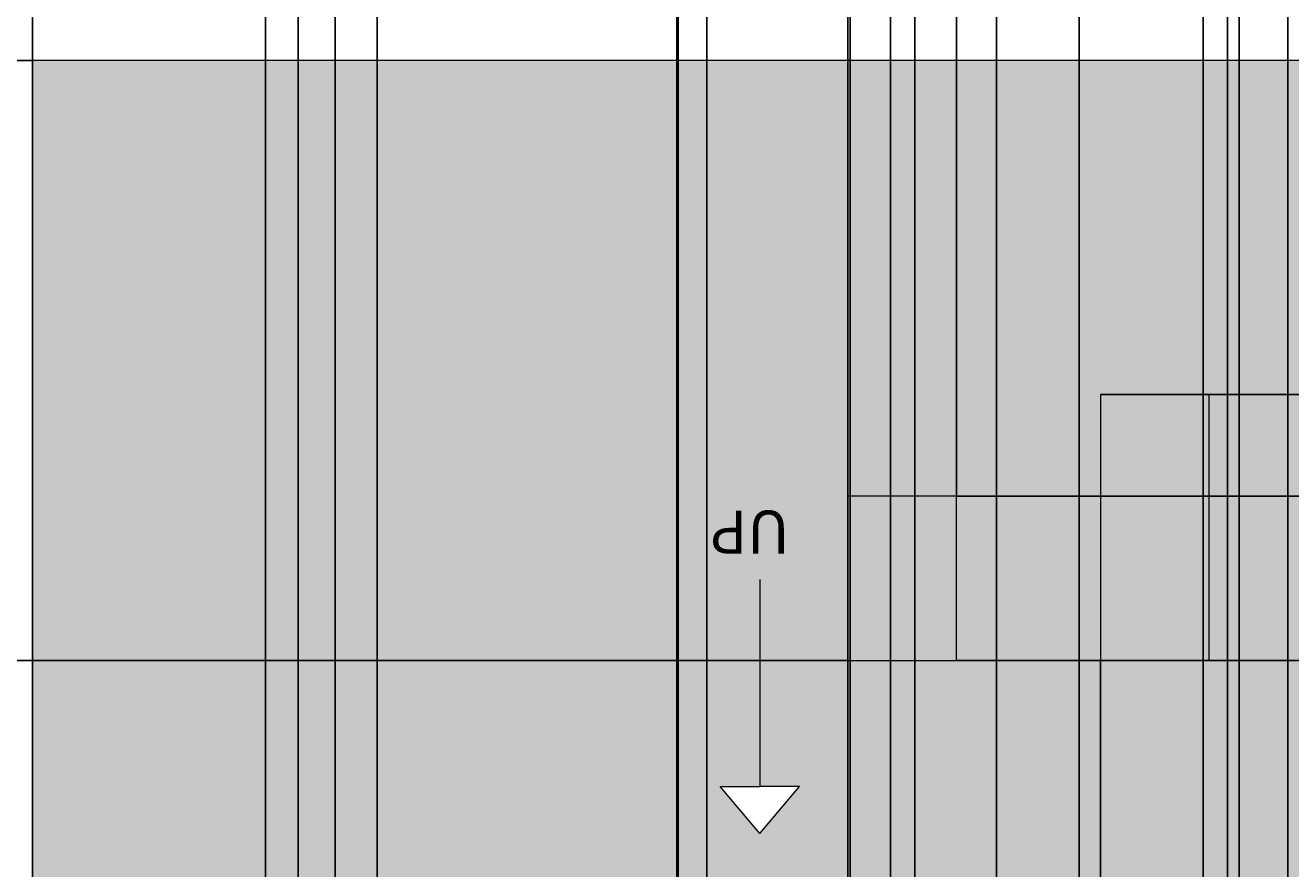
# Model space of a CAD drawing. Units: inches. Extents: x 818 to 1898, y 976 to 2364.
# Tile 78 of 96: x 1083 to 1259, y 2093 to 2211. Entities that reach past the tile are written whole.
import ezdxf

# ---------------------------------------------------------------- set-up
doc = ezdxf.new("R2010")
doc.units = ezdxf.units.IN
doc.header["$LTSCALE"] = 5
doc.header["$MEASUREMENT"] = 0
for name, color, linetype, lineweight in [('A-ANNO-DIMS', 2, 'Continuous', 18), ('A-ANNO-SYMB', 7, 'Continuous', 18), ('A-ANNO-TEXT', 7, 'Continuous', 18), ('L-PAVE', 8, 'Continuous', 18), ('L-PLNT-BEDS', 94, 'Continuous', 18)]:
    doc.layers.add(name, color=color, linetype=linetype, lineweight=lineweight)
doc.layers.add('L-PAVE-PATT', color=9, linetype='Continuous', lineweight=9, true_color=0xc7c8ca)
doc.layers.add('L-PLNT-PATT', color=114, linetype='Continuous', lineweight=9, true_color=0x139b48)
doc.styles.get("Standard").update_dxf_attribs({"font": 'arial.ttf'})
doc.dimstyles.get("Standard").update_dxf_attribs({"dimtxt": 0.18, "dimasz": 0.18, "dimexe": 0.18, "dimexo": 0.0625, "dimgap": 0.09, "dimtad": 0, "dimtih": 1, "dimtoh": 1, "dimdec": 4, "dimzin": 0, "dimdsep": 46, "dimtxsty": 'Standard', "dimcen": 0.09, "dimadec": 0, "dimazin": 0, "dimtfac": 1, "dimtdec": 4, "dimtofl": 0, "dimtmove": 0, "dimatfit": 3, "dimfxl": 1, "dimtolj": 1, "dimtzin": 0, "dimarcsym": 0})

# ---------------------------------------------------------------- blocks, each defined once
blk = doc.blocks.new('*D59')
at = {"layer": 'A-ANNO-DIMS', "color": 0, "lineweight": -2, "ltscale": 5, "transparency": 16777216}
for p, q in [((1251.64, 2300.39), (818.03, 2300.39)), ((818.21, 2300.21), (818.21, 1669.95)), ((818.21, 1039.32), (818.21, 1669.59)), ((896.05, 1039.14), (818.03, 1039.14))]:
    blk.add_line(p, q, dxfattribs=at)
at = {"layer": 'A-ANNO-DIMS', "color": 0, "ltscale": 5, "transparency": 16777216}
for points in [[(818.18, 2300.21), (818.24, 2300.21), (818.21, 2300.39)], [(818.18, 1039.32), (818.24, 1039.32), (818.21, 1039.14)]]:
    blk.add_solid(points, dxfattribs=at)
at = {"layer": 'Defpoints', "color": 0, "ltscale": 5, "transparency": 16777216}
for p in [(818.21, 2300.39), (1251.71, 2300.39), (896.11, 1039.14)]:
    blk.add_point(p, dxfattribs=at)
at = {"layer": 'A-ANNO-DIMS', "color": 0, "ltscale": 5, "transparency": 16777216, "insert": (818.21, 1669.77), "char_height": 0.18, "attachment_point": 5}
blk.add_mtext('\\A1;1261.2', dxfattribs=at)
blk = doc.blocks.new('*D61')
at = {"layer": 'A-ANNO-DIMS', "color": 0, "lineweight": -2, "ltscale": 5, "transparency": 16777216}
for p, q in [((1071.73, 1203.03), (1071.73, 2363.87)), ((1071.91, 2363.69), (1250.94, 2363.69)), ((1430.55, 2363.69), (1251.51, 2363.69)), ((1430.73, 1203.03), (1430.73, 2363.87))]:
    blk.add_line(p, q, dxfattribs=at)
at = {"layer": 'A-ANNO-DIMS', "color": 0, "ltscale": 5, "transparency": 16777216}
for points in [[(1071.91, 2363.72), (1071.91, 2363.66), (1071.73, 2363.69)], [(1430.55, 2363.72), (1430.55, 2363.66), (1430.73, 2363.69)]]:
    blk.add_solid(points, dxfattribs=at)
at = {"layer": 'Defpoints', "color": 0, "ltscale": 5, "transparency": 16777216}
for p in [(1430.73, 2363.69), (1071.73, 1202.96), (1430.73, 1202.96)]:
    blk.add_point(p, dxfattribs=at)
at = {"layer": 'A-ANNO-DIMS', "color": 0, "ltscale": 5, "transparency": 16777216, "insert": (1251.23, 2363.69), "char_height": 0.18, "attachment_point": 5}
blk.add_mtext('\\A1;359', dxfattribs=at)
blk = doc.blocks.new('*D64')
at = {"layer": 'A-ANNO-DIMS', "color": 0, "lineweight": -2, "ltscale": 5, "transparency": 16777216}
for p, q in [((1197.73, 1501.14), (1197.73, 2363.87)), ((1197.91, 2363.69), (1313.93, 2363.69)), ((1430.55, 2363.69), (1314.52, 2363.69)), ((1430.73, 1501.14), (1430.73, 2363.87))]:
    blk.add_line(p, q, dxfattribs=at)
at = {"layer": 'A-ANNO-DIMS', "color": 0, "ltscale": 5, "transparency": 16777216}
for points in [[(1197.91, 2363.72), (1197.91, 2363.66), (1197.73, 2363.69)], [(1430.55, 2363.72), (1430.55, 2363.66), (1430.73, 2363.69)]]:
    blk.add_solid(points, dxfattribs=at)
at = {"layer": 'Defpoints', "color": 0, "ltscale": 5, "transparency": 16777216}
for p in [(1430.73, 2363.69), (1197.73, 1501.08), (1430.73, 1501.08)]:
    blk.add_point(p, dxfattribs=at)
at = {"layer": 'A-ANNO-DIMS', "color": 0, "ltscale": 5, "transparency": 16777216, "insert": (1314.23, 2363.69), "char_height": 0.18, "attachment_point": 5}
blk.add_mtext('\\A1;233', dxfattribs=at)
blk = doc.blocks.new('*D67')
at = {"layer": 'A-ANNO-DIMS', "color": 0, "lineweight": -2, "ltscale": 5, "transparency": 16777216}
for p, q in [((1083.66, 2205.97), (818.03, 2205.97)), ((818.21, 2205.79), (818.21, 2129.71)), ((818.21, 2053.26), (818.21, 2129.34)), ((1083.66, 2053.08), (818.03, 2053.08))]:
    blk.add_line(p, q, dxfattribs=at)
at = {"layer": 'A-ANNO-DIMS', "color": 0, "ltscale": 5, "transparency": 16777216}
for points in [[(818.18, 2205.79), (818.24, 2205.79), (818.21, 2205.97)], [(818.18, 2053.26), (818.24, 2053.26), (818.21, 2053.08)]]:
    blk.add_solid(points, dxfattribs=at)
at = {"layer": 'Defpoints', "color": 0, "ltscale": 5, "transparency": 16777216}
for p in [(818.21, 2205.97), (1083.73, 2205.97), (1083.73, 2053.08)]:
    blk.add_point(p, dxfattribs=at)
at = {"layer": 'A-ANNO-DIMS', "color": 0, "ltscale": 5, "transparency": 16777216, "insert": (818.21, 2129.52), "char_height": 0.18, "attachment_point": 5}
blk.add_mtext('\\A1;152.9', dxfattribs=at)
blk = doc.blocks.new('*D82')
at = {"layer": 'A-ANNO-DIMS', "color": 0, "lineweight": -2, "ltscale": 5, "transparency": 16777216}
for p, q in [((1083.73, 1501.14), (1083.73, 2363.87)), ((1083.91, 2363.69), (1140.45, 2363.69)), ((1197.55, 2363.69), (1141.01, 2363.69)), ((1197.73, 1501.14), (1197.73, 2363.87))]:
    blk.add_line(p, q, dxfattribs=at)
at = {"layer": 'A-ANNO-DIMS', "color": 0, "ltscale": 5, "transparency": 16777216}
for points in [[(1083.91, 2363.72), (1083.91, 2363.66), (1083.73, 2363.69)], [(1197.55, 2363.72), (1197.55, 2363.66), (1197.73, 2363.69)]]:
    blk.add_solid(points, dxfattribs=at)
at = {"layer": 'Defpoints', "color": 0, "ltscale": 5, "transparency": 16777216}
for p in [(1197.73, 2363.69), (1083.73, 1501.08), (1197.73, 1501.08)]:
    blk.add_point(p, dxfattribs=at)
at = {"layer": 'A-ANNO-DIMS', "color": 0, "ltscale": 5, "transparency": 16777216, "insert": (1140.73, 2363.69), "char_height": 0.18, "attachment_point": 5}
blk.add_mtext('\\A1;114', dxfattribs=at)
blk = doc.blocks.new('*D83')
at = {"layer": 'A-ANNO-DIMS', "color": 0, "lineweight": -2, "ltscale": 5, "transparency": 16777216}
for p, q in [((1197.73, 1700.14), (1197.73, 2363.87)), ((1197.91, 2363.69), (1228.02, 2363.69)), ((1258.55, 2363.69), (1228.43, 2363.69)), ((1258.73, 1700.14), (1258.73, 2363.87))]:
    blk.add_line(p, q, dxfattribs=at)
at = {"layer": 'A-ANNO-DIMS', "color": 0, "ltscale": 5, "transparency": 16777216}
for points in [[(1197.91, 2363.72), (1197.91, 2363.66), (1197.73, 2363.69)], [(1258.55, 2363.72), (1258.55, 2363.66), (1258.73, 2363.69)]]:
    blk.add_solid(points, dxfattribs=at)
at = {"layer": 'Defpoints', "color": 0, "ltscale": 5, "transparency": 16777216}
for p in [(1258.73, 2363.69), (1197.73, 1700.08), (1258.73, 1700.08)]:
    blk.add_point(p, dxfattribs=at)
at = {"layer": 'A-ANNO-DIMS', "color": 0, "ltscale": 5, "transparency": 16777216, "insert": (1228.23, 2363.69), "char_height": 0.18, "attachment_point": 5}
blk.add_mtext('\\A1;61', dxfattribs=at)
blk = doc.blocks.new('*D86')
at = {"layer": 'A-ANNO-DIMS', "color": 0, "lineweight": -2, "ltscale": 5, "transparency": 16777216}
for p, q in [((1258.73, 2053.14), (1258.73, 2363.87)), ((1258.91, 2363.69), (1486.43, 2363.69)), ((1714.55, 2363.69), (1487.02, 2363.69)), ((1714.73, 2053.14), (1714.73, 2363.87))]:
    blk.add_line(p, q, dxfattribs=at)
at = {"layer": 'A-ANNO-DIMS', "color": 0, "ltscale": 5, "transparency": 16777216}
for points in [[(1258.91, 2363.72), (1258.91, 2363.66), (1258.73, 2363.69)], [(1714.55, 2363.72), (1714.55, 2363.66), (1714.73, 2363.69)]]:
    blk.add_solid(points, dxfattribs=at)
at = {"layer": 'Defpoints', "color": 0, "ltscale": 5, "transparency": 16777216}
for p in [(1714.73, 2363.69), (1258.73, 2053.08), (1714.73, 2053.08)]:
    blk.add_point(p, dxfattribs=at)
at = {"layer": 'A-ANNO-DIMS', "color": 0, "ltscale": 5, "transparency": 16777216, "insert": (1486.73, 2363.69), "char_height": 0.18, "attachment_point": 5}
blk.add_mtext('\\A1;456', dxfattribs=at)
blk = doc.blocks.new('*D87')
at = {"layer": 'A-ANNO-DIMS', "color": 0, "lineweight": -2, "ltscale": 5, "transparency": 16777216}
for p, q in [((992.73, 2294.28), (992.73, 2363.87)), ((992.91, 2363.69), (1038.02, 2363.69)), ((1083.55, 2363.69), (1038.43, 2363.69)), ((1083.73, 2206.03), (1083.73, 2363.87))]:
    blk.add_line(p, q, dxfattribs=at)
at = {"layer": 'A-ANNO-DIMS', "color": 0, "ltscale": 5, "transparency": 16777216}
for points in [[(992.91, 2363.72), (992.91, 2363.66), (992.73, 2363.69)], [(1083.55, 2363.72), (1083.55, 2363.66), (1083.73, 2363.69)]]:
    blk.add_solid(points, dxfattribs=at)
at = {"layer": 'Defpoints', "color": 0, "ltscale": 5, "transparency": 16777216}
for p in [(1083.73, 2363.69), (992.73, 2294.22), (1083.73, 2205.97)]:
    blk.add_point(p, dxfattribs=at)
at = {"layer": 'A-ANNO-DIMS', "color": 0, "ltscale": 5, "transparency": 16777216, "insert": (1038.23, 2363.69), "char_height": 0.18, "attachment_point": 5}
blk.add_mtext('\\A1;91', dxfattribs=at)
blk = doc.blocks.new('*D93')
at = {"layer": 'A-ANNO-DIMS', "color": 0, "lineweight": -2, "ltscale": 5, "transparency": 16777216}
for p, q in [((1068.34, 1071.12), (1068.34, 2363.87)), ((1068.52, 2363.69), (1094.16, 2363.69)), ((1120.58, 2363.69), (1094.94, 2363.69)), ((1120.76, 1071.12), (1120.76, 2363.87))]:
    blk.add_line(p, q, dxfattribs=at)
at = {"layer": 'A-ANNO-DIMS', "color": 0, "ltscale": 5, "transparency": 16777216}
for points in [[(1068.52, 2363.72), (1068.52, 2363.66), (1068.34, 2363.69)], [(1120.58, 2363.72), (1120.58, 2363.66), (1120.76, 2363.69)]]:
    blk.add_solid(points, dxfattribs=at)
at = {"layer": 'Defpoints', "color": 0, "ltscale": 5, "transparency": 16777216}
for p in [(1120.76, 2363.69), (1068.34, 1071.06), (1120.76, 1071.06)]:
    blk.add_point(p, dxfattribs=at)
at = {"layer": 'A-ANNO-DIMS', "color": 0, "ltscale": 5, "transparency": 16777216, "insert": (1094.55, 2363.69), "char_height": 0.18, "attachment_point": 5}
blk.add_mtext('\\A1;52.42', dxfattribs=at)
blk = doc.blocks.new('*D94')
at = {"layer": 'A-ANNO-DIMS', "color": 0, "lineweight": -2, "ltscale": 5, "transparency": 16777216}
for p, q in [((1120.76, 1071.12), (1120.76, 2363.87)), ((1120.94, 2363.69), (1146.76, 2363.69)), ((1173.36, 2363.69), (1147.55, 2363.69)), ((1173.54, 1071.12), (1173.54, 2363.87))]:
    blk.add_line(p, q, dxfattribs=at)
at = {"layer": 'A-ANNO-DIMS', "color": 0, "ltscale": 5, "transparency": 16777216}
for points in [[(1120.94, 2363.72), (1120.94, 2363.66), (1120.76, 2363.69)], [(1173.36, 2363.72), (1173.36, 2363.66), (1173.54, 2363.69)]]:
    blk.add_solid(points, dxfattribs=at)
at = {"layer": 'Defpoints', "color": 0, "ltscale": 5, "transparency": 16777216}
for p in [(1173.54, 2363.69), (1120.76, 1071.06), (1173.54, 1071.06)]:
    blk.add_point(p, dxfattribs=at)
at = {"layer": 'A-ANNO-DIMS', "color": 0, "ltscale": 5, "transparency": 16777216, "insert": (1147.15, 2363.69), "char_height": 0.18, "attachment_point": 5}
blk.add_mtext('\\A1;52.78', dxfattribs=at)
blk = doc.blocks.new('*D95')
at = {"layer": 'A-ANNO-DIMS', "color": 0, "lineweight": -2, "ltscale": 5, "transparency": 16777216}
for p, q in [((1173.54, 1071.12), (1173.54, 2363.87)), ((1173.72, 2363.69), (1201.29, 2363.69)), ((1229.47, 2363.69), (1201.9, 2363.69)), ((1229.65, 1071.12), (1229.65, 2363.87))]:
    blk.add_line(p, q, dxfattribs=at)
at = {"layer": 'A-ANNO-DIMS', "color": 0, "ltscale": 5, "transparency": 16777216}
for points in [[(1173.72, 2363.72), (1173.72, 2363.66), (1173.54, 2363.69)], [(1229.47, 2363.72), (1229.47, 2363.66), (1229.65, 2363.69)]]:
    blk.add_solid(points, dxfattribs=at)
at = {"layer": 'Defpoints', "color": 0, "ltscale": 5, "transparency": 16777216}
for p in [(1229.65, 2363.69), (1173.54, 1071.06), (1229.65, 1071.06)]:
    blk.add_point(p, dxfattribs=at)
at = {"layer": 'A-ANNO-DIMS', "color": 0, "ltscale": 5, "transparency": 16777216, "insert": (1201.59, 2363.69), "char_height": 0.18, "attachment_point": 5}
blk.add_mtext('\\A1;56.1', dxfattribs=at)
blk = doc.blocks.new('*D96')
at = {"layer": 'A-ANNO-DIMS', "color": 0, "lineweight": -2, "ltscale": 5, "transparency": 16777216}
for p, q in [((1229.65, 1071.12), (1229.65, 2363.87)), ((1229.83, 2363.69), (1256.52, 2363.69)), ((1283.99, 2363.69), (1257.3, 2363.69)), ((1284.17, 1071.12), (1284.17, 2363.87))]:
    blk.add_line(p, q, dxfattribs=at)
at = {"layer": 'A-ANNO-DIMS', "color": 0, "ltscale": 5, "transparency": 16777216}
for points in [[(1229.83, 2363.72), (1229.83, 2363.66), (1229.65, 2363.69)], [(1283.99, 2363.72), (1283.99, 2363.66), (1284.17, 2363.69)]]:
    blk.add_solid(points, dxfattribs=at)
at = {"layer": 'Defpoints', "color": 0, "ltscale": 5, "transparency": 16777216}
for p in [(1284.17, 2363.69), (1229.65, 1071.06), (1284.17, 1071.06)]:
    blk.add_point(p, dxfattribs=at)
at = {"layer": 'A-ANNO-DIMS', "color": 0, "ltscale": 5, "transparency": 16777216, "insert": (1256.91, 2363.69), "char_height": 0.18, "attachment_point": 5}
blk.add_mtext('\\A1;54.52', dxfattribs=at)
blk = doc.blocks.new('*D109')
at = {"layer": 'A-ANNO-DIMS', "color": 0, "lineweight": -2, "ltscale": 5, "transparency": 16777216}
for p, q in [((1125.92, 1410.12), (1125.92, 2363.87)), ((1126.1, 2363.69), (1164.25, 2363.69)), ((1203.15, 2363.69), (1165, 2363.69)), ((1203.33, 1409.91), (1203.33, 2363.87))]:
    blk.add_line(p, q, dxfattribs=at)
at = {"layer": 'A-ANNO-DIMS', "color": 0, "ltscale": 5, "transparency": 16777216}
for points in [[(1126.1, 2363.72), (1126.1, 2363.66), (1125.92, 2363.69)], [(1203.15, 2363.72), (1203.15, 2363.66), (1203.33, 2363.69)]]:
    blk.add_solid(points, dxfattribs=at)
at = {"layer": 'Defpoints', "color": 0, "ltscale": 5, "transparency": 16777216}
for p in [(1203.33, 2363.69), (1125.92, 1410.05), (1203.33, 1409.85)]:
    blk.add_point(p, dxfattribs=at)
at = {"layer": 'A-ANNO-DIMS', "color": 0, "ltscale": 5, "transparency": 16777216, "insert": (1164.62, 2363.69), "char_height": 0.18, "attachment_point": 5}
blk.add_mtext('\\A1;77.41', dxfattribs=at)
blk = doc.blocks.new('*D123')
at = {"layer": 'A-ANNO-DIMS', "color": 0, "lineweight": -2, "ltscale": 5, "transparency": 16777216}
for p, q in [((1083.73, 2044.14), (1083.73, 2363.87)), ((1083.91, 2363.69), (1107.35, 2363.69)), ((1131.59, 2363.69), (1108.14, 2363.69)), ((1131.77, 1974.64), (1131.77, 2363.87))]:
    blk.add_line(p, q, dxfattribs=at)
at = {"layer": 'A-ANNO-DIMS', "color": 0, "ltscale": 5, "transparency": 16777216}
for points in [[(1083.91, 2363.72), (1083.91, 2363.66), (1083.73, 2363.69)], [(1131.59, 2363.72), (1131.59, 2363.66), (1131.77, 2363.69)]]:
    blk.add_solid(points, dxfattribs=at)
at = {"layer": 'Defpoints', "color": 0, "ltscale": 5, "transparency": 16777216}
for p in [(1131.77, 2363.69), (1083.73, 2044.08), (1131.77, 1974.57)]:
    blk.add_point(p, dxfattribs=at)
at = {"layer": 'A-ANNO-DIMS', "color": 0, "ltscale": 5, "transparency": 16777216, "insert": (1107.75, 2363.69), "char_height": 0.18, "attachment_point": 5}
blk.add_mtext('\\A1;48.04', dxfattribs=at)
blk = doc.blocks.new('*D126')
at = {"layer": 'A-ANNO-DIMS', "color": 0, "lineweight": -2, "ltscale": 5, "transparency": 16777216}
for p, q in [((1035.38, 1252.09), (1035.38, 2363.87)), ((1035.56, 2363.69), (1075.41, 2363.69)), ((1116.01, 2363.69), (1076.16, 2363.69)), ((1116.19, 1236.03), (1116.19, 2363.87))]:
    blk.add_line(p, q, dxfattribs=at)
at = {"layer": 'A-ANNO-DIMS', "color": 0, "ltscale": 5, "transparency": 16777216}
for points in [[(1035.56, 2363.72), (1035.56, 2363.66), (1035.38, 2363.69)], [(1116.01, 2363.72), (1116.01, 2363.66), (1116.19, 2363.69)]]:
    blk.add_solid(points, dxfattribs=at)
at = {"layer": 'Defpoints', "color": 0, "ltscale": 5, "transparency": 16777216}
for p in [(1035.38, 2363.69), (1035.38, 1252.02), (1116.19, 1235.96)]:
    blk.add_point(p, dxfattribs=at)
at = {"layer": 'A-ANNO-DIMS', "color": 0, "ltscale": 5, "transparency": 16777216, "insert": (1075.78, 2363.69), "char_height": 0.18, "attachment_point": 5}
blk.add_mtext('\\A1;80.81', dxfattribs=at)
blk = doc.blocks.new('*D140')
at = {"layer": 'A-ANNO-DIMS', "color": 0, "lineweight": -2, "ltscale": 5, "transparency": 16777216}
for p, q in [((1083.73, 2053.14), (1083.73, 2363.87)), ((1083.91, 2363.69), (1150.46, 2363.69)), ((1217.93, 2363.69), (1151.37, 2363.69)), ((1218.11, 2083.32), (1218.11, 2363.87))]:
    blk.add_line(p, q, dxfattribs=at)
at = {"layer": 'A-ANNO-DIMS', "color": 0, "ltscale": 5, "transparency": 16777216}
for points in [[(1083.91, 2363.72), (1083.91, 2363.66), (1083.73, 2363.69)], [(1217.93, 2363.72), (1217.93, 2363.66), (1218.11, 2363.69)]]:
    blk.add_solid(points, dxfattribs=at)
at = {"layer": 'Defpoints', "color": 0, "ltscale": 5, "transparency": 16777216}
for p in [(1218.11, 2363.69), (1218.11, 2083.26), (1083.73, 2053.08)]:
    blk.add_point(p, dxfattribs=at)
at = {"layer": 'A-ANNO-DIMS', "color": 0, "ltscale": 5, "transparency": 16777216, "insert": (1150.92, 2363.69), "char_height": 0.18, "attachment_point": 5}
blk.add_mtext('\\A1;134.39', dxfattribs=at)
blk = doc.blocks.new('*D143')
at = {"layer": 'A-ANNO-DIMS', "color": 0, "lineweight": -2, "ltscale": 5, "transparency": 16777216}
for p, q in [((1083.73, 2206.03), (1083.73, 2363.87)), ((1083.91, 2363.69), (1140.1, 2363.69)), ((1197.21, 2363.69), (1141.01, 2363.69)), ((1197.39, 2122.44), (1197.39, 2363.87))]:
    blk.add_line(p, q, dxfattribs=at)
at = {"layer": 'A-ANNO-DIMS', "color": 0, "ltscale": 5, "transparency": 16777216}
for points in [[(1083.91, 2363.72), (1083.91, 2363.66), (1083.73, 2363.69)], [(1197.21, 2363.72), (1197.21, 2363.66), (1197.39, 2363.69)]]:
    blk.add_solid(points, dxfattribs=at)
at = {"layer": 'Defpoints', "color": 0, "ltscale": 5, "transparency": 16777216}
for p in [(1197.39, 2363.69), (1083.73, 2205.97), (1197.39, 2122.38)]:
    blk.add_point(p, dxfattribs=at)
at = {"layer": 'A-ANNO-DIMS', "color": 0, "ltscale": 5, "transparency": 16777216, "insert": (1140.56, 2363.69), "char_height": 0.18, "attachment_point": 5}
blk.add_mtext('\\A1;113.67', dxfattribs=at)
blk = doc.blocks.new('*D144')
at = {"layer": 'A-ANNO-DIMS', "color": 0, "lineweight": -2, "ltscale": 5, "transparency": 16777216}
for p, q in [((1197.39, 2122.44), (1197.39, 2363.87)), ((1197.57, 2363.69), (1204.5, 2363.69)), ((1212.34, 2363.69), (1205.41, 2363.69)), ((1212.52, 2145.31), (1212.52, 2363.87))]:
    blk.add_line(p, q, dxfattribs=at)
at = {"layer": 'A-ANNO-DIMS', "color": 0, "ltscale": 5, "transparency": 16777216}
for points in [[(1197.57, 2363.72), (1197.57, 2363.66), (1197.39, 2363.69)], [(1212.34, 2363.72), (1212.34, 2363.66), (1212.52, 2363.69)]]:
    blk.add_solid(points, dxfattribs=at)
at = {"layer": 'Defpoints', "color": 0, "ltscale": 5, "transparency": 16777216}
for p in [(1212.52, 2363.69), (1212.52, 2145.25), (1197.39, 2122.38)]:
    blk.add_point(p, dxfattribs=at)
at = {"layer": 'A-ANNO-DIMS', "color": 0, "ltscale": 5, "transparency": 16777216, "insert": (1204.96, 2363.69), "char_height": 0.18, "attachment_point": 5}
blk.add_mtext('\\A1;15.128', dxfattribs=at)
blk = doc.blocks.new('*D145')
at = {"layer": 'A-ANNO-DIMS', "color": 0, "lineweight": -2, "ltscale": 5, "transparency": 16777216}
for p, q in [((1197.39, 2122.31), (1197.39, 975.66)), ((1232.61, 2122.31), (1232.61, 975.66)), ((1197.57, 975.84), (1214.61, 975.84)), ((1232.43, 975.84), (1215.39, 975.84))]:
    blk.add_line(p, q, dxfattribs=at)
at = {"layer": 'A-ANNO-DIMS', "color": 0, "ltscale": 5, "transparency": 16777216}
for points in [[(1197.57, 975.87), (1197.57, 975.81), (1197.39, 975.84)], [(1232.43, 975.87), (1232.43, 975.81), (1232.61, 975.84)]]:
    blk.add_solid(points, dxfattribs=at)
at = {"layer": 'Defpoints', "color": 0, "ltscale": 5, "transparency": 16777216}
for p in [(1197.39, 2122.38), (1232.61, 2122.38), (1232.61, 975.84)]:
    blk.add_point(p, dxfattribs=at)
at = {"layer": 'A-ANNO-DIMS', "color": 0, "ltscale": 5, "transparency": 16777216, "insert": (1215, 975.84), "char_height": 0.18, "attachment_point": 5}
blk.add_mtext('\\A1;35.22', dxfattribs=at)
blk = doc.blocks.new('*D146')
at = {"layer": 'A-ANNO-DIMS', "color": 0, "lineweight": -2, "ltscale": 5, "transparency": 16777216}
for p, q in [((1197.33, 2122.38), (818.03, 2122.38)), ((818.21, 2122.2), (818.21, 2087.91)), ((818.21, 2053.26), (818.21, 2087.55)), ((1083.66, 2053.08), (818.03, 2053.08))]:
    blk.add_line(p, q, dxfattribs=at)
at = {"layer": 'A-ANNO-DIMS', "color": 0, "ltscale": 5, "transparency": 16777216}
for points in [[(818.18, 2122.2), (818.24, 2122.2), (818.21, 2122.38)], [(818.18, 2053.26), (818.24, 2053.26), (818.21, 2053.08)]]:
    blk.add_solid(points, dxfattribs=at)
at = {"layer": 'Defpoints', "color": 0, "ltscale": 5, "transparency": 16777216}
for p in [(1197.39, 2122.38), (818.21, 2053.08), (1083.73, 2053.08)]:
    blk.add_point(p, dxfattribs=at)
at = {"layer": 'A-ANNO-DIMS', "color": 0, "ltscale": 5, "transparency": 16777216, "insert": (818.21, 2087.73), "char_height": 0.18, "attachment_point": 5}
blk.add_mtext('\\A1;69.3', dxfattribs=at)
blk = doc.blocks.new('*D147')
at = {"layer": 'A-ANNO-DIMS', "color": 0, "lineweight": -2, "ltscale": 5, "transparency": 16777216}
for p, q in [((1212.58, 2145.25), (1897.92, 2145.25)), ((1897.74, 2145.07), (1897.74, 2133.99)), ((1897.74, 2122.56), (1897.74, 2133.63)), ((1212.58, 2122.38), (1897.92, 2122.38))]:
    blk.add_line(p, q, dxfattribs=at)
at = {"layer": 'A-ANNO-DIMS', "color": 0, "ltscale": 5, "transparency": 16777216}
for points in [[(1897.71, 2145.07), (1897.77, 2145.07), (1897.74, 2145.25)], [(1897.71, 2122.56), (1897.77, 2122.56), (1897.74, 2122.38)]]:
    blk.add_solid(points, dxfattribs=at)
at = {"layer": 'Defpoints', "color": 0, "ltscale": 5, "transparency": 16777216}
for p in [(1212.52, 2145.25), (1897.74, 2145.25), (1212.52, 2122.38)]:
    blk.add_point(p, dxfattribs=at)
at = {"layer": 'A-ANNO-DIMS', "color": 0, "ltscale": 5, "transparency": 16777216, "insert": (1897.74, 2133.81), "char_height": 0.18, "attachment_point": 5}
blk.add_mtext('\\A1;22.87', dxfattribs=at)
blk = doc.blocks.new('*D148')
at = {"layer": 'A-ANNO-DIMS', "color": 0, "lineweight": -2, "ltscale": 5, "transparency": 16777216}
for p, q in [((1232.67, 2159.43), (1897.92, 2159.43)), ((1897.74, 2159.25), (1897.74, 2141.09)), ((1897.74, 2122.56), (1897.74, 2140.72)), ((1232.67, 2122.38), (1897.92, 2122.38))]:
    blk.add_line(p, q, dxfattribs=at)
at = {"layer": 'A-ANNO-DIMS', "color": 0, "ltscale": 5, "transparency": 16777216}
for points in [[(1897.71, 2159.25), (1897.77, 2159.25), (1897.74, 2159.43)], [(1897.71, 2122.56), (1897.77, 2122.56), (1897.74, 2122.38)]]:
    blk.add_solid(points, dxfattribs=at)
at = {"layer": 'Defpoints', "color": 0, "ltscale": 5, "transparency": 16777216}
for p in [(1232.61, 2159.43), (1897.74, 2159.43), (1232.61, 2122.38)]:
    blk.add_point(p, dxfattribs=at)
at = {"layer": 'A-ANNO-DIMS', "color": 0, "ltscale": 5, "transparency": 16777216, "insert": (1897.74, 2140.9), "char_height": 0.18, "attachment_point": 5}
blk.add_mtext('\\A1;37.05', dxfattribs=at)
blk = doc.blocks.new('*D158')
at = {"layer": 'A-ANNO-DIMS', "color": 0, "lineweight": -2, "ltscale": 5, "transparency": 16777216}
for p, q in [((1173.73, 1590.82), (1173.73, 2363.87)), ((1173.91, 2363.69), (1175.57, 2363.69)), ((1177.55, 2363.69), (1175.88, 2363.69)), ((1177.73, 1586.82), (1177.73, 2363.87))]:
    blk.add_line(p, q, dxfattribs=at)
at = {"layer": 'A-ANNO-DIMS', "color": 0, "ltscale": 5, "transparency": 16777216}
for points in [[(1173.91, 2363.72), (1173.91, 2363.66), (1173.73, 2363.69)], [(1177.55, 2363.72), (1177.55, 2363.66), (1177.73, 2363.69)]]:
    blk.add_solid(points, dxfattribs=at)
at = {"layer": 'Defpoints', "color": 0, "ltscale": 5, "transparency": 16777216}
for p in [(1177.73, 2363.69), (1173.73, 1590.76), (1177.73, 1586.76)]:
    blk.add_point(p, dxfattribs=at)
at = {"layer": 'A-ANNO-DIMS', "color": 0, "ltscale": 5, "transparency": 16777216, "insert": (1175.73, 2363.69), "char_height": 0.18, "attachment_point": 5}
blk.add_mtext('\\A1;4', dxfattribs=at)
blk = doc.blocks.new('*D269')
at = {"layer": 'A-ANNO-DIMS', "color": 0, "lineweight": -2, "ltscale": 5, "transparency": 16777216}
for p, q in [((1246.94, 1534.14), (1246.94, 2363.87)), ((1247.12, 2363.69), (1293.71, 2363.69)), ((1341.08, 2363.69), (1294.49, 2363.69)), ((1341.26, 1534.14), (1341.26, 2363.87))]:
    blk.add_line(p, q, dxfattribs=at)
at = {"layer": 'A-ANNO-DIMS', "color": 0, "ltscale": 5, "transparency": 16777216}
for points in [[(1247.12, 2363.72), (1247.12, 2363.66), (1246.94, 2363.69)], [(1341.08, 2363.72), (1341.08, 2363.66), (1341.26, 2363.69)]]:
    blk.add_solid(points, dxfattribs=at)
at = {"layer": 'Defpoints', "color": 0, "ltscale": 5, "transparency": 16777216}
for p in [(1341.26, 2363.69), (1246.94, 1534.08), (1341.26, 1534.08)]:
    blk.add_point(p, dxfattribs=at)
at = {"layer": 'A-ANNO-DIMS', "color": 0, "ltscale": 5, "transparency": 16777216, "insert": (1294.1, 2363.69), "char_height": 0.18, "attachment_point": 5}
blk.add_mtext('\\A1;94.32', dxfattribs=at)
blk = doc.blocks.new('*D271')
at = {"layer": 'A-ANNO-DIMS', "color": 0, "lineweight": -2, "ltscale": 5, "transparency": 16777216}
for p, q in [((1206.73, 1510.14), (1206.73, 2363.87)), ((1206.91, 2363.69), (1226.45, 2363.69)), ((1246.76, 2363.69), (1227.21, 2363.69)), ((1246.94, 1510.14), (1246.94, 2363.87))]:
    blk.add_line(p, q, dxfattribs=at)
at = {"layer": 'A-ANNO-DIMS', "color": 0, "ltscale": 5, "transparency": 16777216}
for points in [[(1206.91, 2363.72), (1206.91, 2363.66), (1206.73, 2363.69)], [(1246.76, 2363.72), (1246.76, 2363.66), (1246.94, 2363.69)]]:
    blk.add_solid(points, dxfattribs=at)
at = {"layer": 'Defpoints', "color": 0, "ltscale": 5, "transparency": 16777216}
for p in [(1246.94, 2363.69), (1206.73, 1510.08), (1246.94, 1510.08)]:
    blk.add_point(p, dxfattribs=at)
at = {"layer": 'A-ANNO-DIMS', "color": 0, "ltscale": 5, "transparency": 16777216, "insert": (1226.83, 2363.69), "char_height": 0.18, "attachment_point": 5}
blk.add_mtext('\\A1;40.21', dxfattribs=at)
blk = doc.blocks.new('*D276')
at = {"layer": 'A-ANNO-DIMS', "color": 0, "lineweight": -2, "ltscale": 5, "transparency": 16777216}
for p, q in [((1206.73, 1687.14), (1206.73, 2363.87)), ((1206.91, 2363.69), (1228.95, 2363.69)), ((1251.75, 2363.69), (1229.71, 2363.69)), ((1251.93, 1681.44), (1251.93, 2363.87))]:
    blk.add_line(p, q, dxfattribs=at)
at = {"layer": 'A-ANNO-DIMS', "color": 0, "ltscale": 5, "transparency": 16777216}
for points in [[(1206.91, 2363.72), (1206.91, 2363.66), (1206.73, 2363.69)], [(1251.75, 2363.72), (1251.75, 2363.66), (1251.93, 2363.69)]]:
    blk.add_solid(points, dxfattribs=at)
at = {"layer": 'Defpoints', "color": 0, "ltscale": 5, "transparency": 16777216}
for p in [(1251.93, 2363.69), (1206.73, 1687.08), (1251.93, 1681.38)]:
    blk.add_point(p, dxfattribs=at)
at = {"layer": 'A-ANNO-DIMS', "color": 0, "ltscale": 5, "transparency": 16777216, "insert": (1229.33, 2363.69), "char_height": 0.18, "attachment_point": 5}
blk.add_mtext('\\A1;45.21', dxfattribs=at)
blk = doc.blocks.new('*D281')
at = {"layer": 'A-ANNO-DIMS', "color": 0, "lineweight": -2, "ltscale": 5, "transparency": 16777216}
for p, q in [((1250.3, 1913.7), (1250.3, 2363.87)), ((1250.48, 2363.69), (1420.12, 2363.69)), ((1590.55, 2363.69), (1420.91, 2363.69)), ((1590.73, 2011.14), (1590.73, 2363.87))]:
    blk.add_line(p, q, dxfattribs=at)
at = {"layer": 'A-ANNO-DIMS', "color": 0, "ltscale": 5, "transparency": 16777216}
for points in [[(1250.48, 2363.72), (1250.48, 2363.66), (1250.3, 2363.69)], [(1590.55, 2363.72), (1590.55, 2363.66), (1590.73, 2363.69)]]:
    blk.add_solid(points, dxfattribs=at)
at = {"layer": 'Defpoints', "color": 0, "ltscale": 5, "transparency": 16777216}
for p in [(1590.73, 2363.69), (1590.73, 2011.08), (1250.3, 1913.64)]:
    blk.add_point(p, dxfattribs=at)
at = {"layer": 'A-ANNO-DIMS', "color": 0, "ltscale": 5, "transparency": 16777216, "insert": (1420.51, 2363.69), "char_height": 0.18, "attachment_point": 5}
blk.add_mtext('\\A1;340.4', dxfattribs=at)

msp = doc.modelspace()

# ---------------------------------------------------------------- hatches: boundary and pattern name
at = {"layer": 'L-PAVE-PATT', "ltscale": 5}
h = msp.add_hatch(color=256, dxfattribs=at)
h.dxf.hatch_style = 1
h.paths.add_polyline_path([(1212.5206, 2145.2461), (1197.3925, 2145.2461), (1197.3925, 2122.3767), (1212.5206, 2122.3767)])
h.paths.add_polyline_path([(1247.7373, 2159.4296), (1232.6091, 2159.4296), (1232.6091, 2122.3767), (1247.7373, 2122.3767)])
h.paths.add_polyline_path([(1282.9539, 2145.2461), (1267.8258, 2145.2461), (1267.8258, 2122.3767), (1282.9539, 2122.3767)])
h.paths.add_polyline_path([(1318.1705, 2145.2461), (1303.0424, 2145.2461), (1303.0424, 2122.3767), (1318.1705, 2122.3767)])
h.paths.add_polyline_path([(1353.3871, 2155.7839), (1338.259, 2155.7839), (1338.259, 2122.3767), (1353.3871, 2122.3767)])
h.paths.add_polyline_path([(1388.6037, 2145.2461), (1373.4756, 2145.2461), (1373.4756, 2122.3767), (1388.6037, 2122.3767)])
h.paths.add_polyline_path([(1423.8203, 2145.2461), (1408.6922, 2145.2461), (1408.6922, 2122.3767), (1423.8203, 2122.3767)])
h.paths.add_polyline_path([(1459.037, 2158.4222), (1443.9089, 2158.4222), (1443.9089, 2122.3767), (1459.037, 2122.3767)])
h.paths.add_polyline_path([(1494.2536, 2145.2461), (1479.1255, 2145.2461), (1479.1255, 2122.3767), (1494.2536, 2122.3767)])
h.paths.add_polyline_path([(1529.4702, 2145.2461), (1514.3421, 2145.2461), (1514.3421, 2122.3767), (1529.4702, 2122.3767)])
h.paths.add_polyline_path([(1564.6868, 2156.9246), (1549.5587, 2156.9246), (1549.5587, 2122.3767), (1564.6868, 2122.3767)])
h.paths.add_polyline_path([(1599.9034, 2145.2461), (1584.7753, 2145.2461), (1584.7753, 2122.3767), (1599.9034, 2122.3767)])
h.paths.add_polyline_path([(1635.1201, 2145.2461), (1619.9919, 2145.2461), (1619.9919, 2122.3767), (1635.1201, 2122.3767)])
h.paths.add_polyline_path([(1670.3367, 2156.1761), (1655.2086, 2156.1761), (1655.2086, 2122.3767), (1670.3367, 2122.3767)])
h.paths.add_polyline_path([(1701.7273, 2145.2461), (1686.5992, 2145.2461), (1686.5992, 2122.3767), (1701.7273, 2122.3767)])
h.paths.add_polyline_path([(1730.8897, 2145.2461), (1715.7616, 2145.2461), (1715.7616, 2122.3767), (1730.8897, 2122.3767)])
h.paths.add_polyline_path([(1776.3312, 2145.2461), (1753.1652, 2145.2461), (1753.1652, 2115.6891), (1776.3312, 2115.6891)])
at = {"layer": 'L-PLNT-PATT', "ltscale": 5}
h = msp.add_hatch(color=256, dxfattribs=at)
h.dxf.hatch_style = 1
h.paths.add_polyline_path([(1789.7173, 2205.9709), (1083.7251, 2205.9709), (1083.7251, 2083.2623), (1218.1114, 2083.2623), (1218.1114, 2053.0782), (1390.6356, 2053.0782), (1390.6356, 2081.1881), (1399.6356, 2081.1881), (1413.02, 2081.1881), (1422.02, 2081.1881), (1422.02, 2053.0782), (1676.6446, 2053.0782), (1676.6446, 2081.1881), (1714.7251, 2081.1881), (1714.7251, 2081.6235), (1789.7173, 2081.6235)])
h.paths.add_polyline_path([(1388.6037, 2145.2461), (1388.6037, 2122.3767), (1373.4756, 2122.3767), (1373.4756, 2145.2461)], flags=16)
h.paths.add_polyline_path([(1408.6922, 2145.2461), (1423.8203, 2145.2461), (1423.8203, 2122.3767), (1408.6922, 2122.3767)], flags=16)
h.paths.add_polyline_path([(1353.3871, 2155.7839), (1353.3871, 2122.3767), (1338.259, 2122.3767), (1338.259, 2155.7839)], flags=16)
h.paths.add_polyline_path([(1443.9089, 2158.4222), (1459.037, 2158.4222), (1459.037, 2122.3767), (1443.9089, 2122.3767)], flags=16)
h.paths.add_polyline_path([(1318.1705, 2145.2461), (1318.1705, 2122.3767), (1303.0424, 2122.3767), (1303.0424, 2145.2461)], flags=16)
h.paths.add_polyline_path([(1479.1255, 2145.2461), (1494.2536, 2145.2461), (1494.2536, 2122.3767), (1479.1255, 2122.3767)], flags=16)
h.paths.add_polyline_path([(1282.9539, 2145.2461), (1282.9539, 2122.3767), (1267.8258, 2122.3767), (1267.8258, 2145.2461)], flags=16)
h.paths.add_polyline_path([(1514.3421, 2145.2461), (1529.4702, 2145.2461), (1529.4702, 2122.3767), (1514.3421, 2122.3767)], flags=16)
h.paths.add_polyline_path([(1247.7373, 2159.4296), (1247.7373, 2122.3767), (1232.6091, 2122.3767), (1232.6091, 2159.4296)], flags=16)
h.paths.add_polyline_path([(1549.5587, 2156.9246), (1564.6868, 2156.9246), (1564.6868, 2122.3767), (1549.5587, 2122.3767)], flags=16)
h.paths.add_polyline_path([(1212.5206, 2145.2461), (1212.5206, 2122.3767), (1197.3925, 2122.3767), (1197.3925, 2145.2461)], flags=16)
h.paths.add_polyline_path([(1584.7753, 2145.2461), (1599.9034, 2145.2461), (1599.9034, 2122.3767), (1584.7753, 2122.3767)], flags=16)
h.paths.add_polyline_path([(1185.1073, 2104.7786), (1190.6407, 2104.7786), (1185.1073, 2098.2505), (1179.5738, 2104.7786)], flags=16)
h.paths.add_polyline_path([(1619.9919, 2145.2461), (1635.1201, 2145.2461), (1635.1201, 2122.3767), (1619.9919, 2122.3767)], flags=16)
h.paths.add_polyline_path([(1655.2086, 2156.1761), (1670.3367, 2156.1761), (1670.3367, 2122.3767), (1655.2086, 2122.3767)], flags=16)
h.paths.add_polyline_path([(1686.5992, 2145.2461), (1701.7273, 2145.2461), (1701.7273, 2122.3767), (1686.5992, 2122.3767)], flags=16)
h.paths.add_polyline_path([(1715.7616, 2145.2461), (1730.8897, 2145.2461), (1730.8897, 2122.3767), (1715.7616, 2122.3767)], flags=16)
h.paths.add_polyline_path([(1753.1652, 2145.2461), (1776.3312, 2145.2461), (1776.3312, 2115.6891), (1753.1652, 2115.6891)], flags=16)
h.paths.add_polyline_path([(1191.4331, 2146.5159), (1176.7891, 2146.5159), (1176.7891, 2134.1516), (1191.4331, 2134.1516)], flags=24)

# ---------------------------------------------------------------- linework, layer by layer
at = {"layer": 'A-ANNO-SYMB', "ltscale": 5}
for p, q in [((1185.1073, 2133.6432), (1185.1073, 2104.7786)), ((1185.1073, 2098.2505), (1179.5738, 2104.7786)), ((1179.5738, 2104.7786), (1185.1073, 2104.7786)), ((1185.1073, 2098.2505), (1190.6407, 2104.7786)), ((1190.6407, 2104.7786), (1185.1073, 2104.7786))]:
    msp.add_line(p, q, dxfattribs=at)
at = {"layer": 'L-PAVE', "ltscale": 5}
for points in [[(1247.7373, 2159.4296), (1232.6091, 2159.4296), (1232.6091, 2122.3767), (1247.7373, 2122.3767)], [(1212.5206, 2145.2461), (1197.3925, 2145.2461), (1197.3925, 2122.3767), (1212.5206, 2122.3767)]]:
    msp.add_lwpolyline(points, close=True, dxfattribs=at)
at = {"layer": 'L-PLNT-BEDS'}
msp.add_line((1083.7251, 2205.9709), (1083.7251, 2053.0782), dxfattribs=at)
at = {"layer": 'L-PLNT-BEDS', "ltscale": 5}
msp.add_line((1789.7173, 2205.9709), (1083.7251, 2205.9709), dxfattribs=at)

# ---------------------------------------------------------------- texts
at = {"layer": 'A-ANNO-TEXT', "ltscale": 5, "insert": (1189.2741, 2137.2396), "char_height": 6, "attachment_point": 1, "rotation": 180}
msp.add_mtext_dynamic_manual_height_columns('UP', width=118.992422, gutter_width=1, heights=[0], dxfattribs=at)

# ---------------------------------------------------------------- dimensions: what is measured, and where the dimension line sits
at = {"layer": 'A-ANNO-DIMS', "ltscale": 5}
for base, p1, p2, override, picture, middle in [((1083.7251, 2363.6929), (992.7251, 2294.2171), (1083.7251, 2205.9709), {"dimdec": 0, "dimlfac": 1, "dimrnd": 0, "dimzin": 0, "dimdsep": 46, "dimlunit": 2}, '*D87', (1038.2251, 2363.6929)), ((1035.3768, 2363.6929), (1116.1882, 1235.9642), (1035.3768, 1252.0242), {"dimdec": 2, "dimlfac": 1, "dimrnd": 0, "dimzin": 0, "dimdsep": 46, "dimlunit": 2}, '*D126', (1075.7825, 2363.6929)), ((1120.7618, 2363.6929), (1068.3377, 1071.0552), (1120.7618, 1071.0552), {"dimdec": 2, "dimlfac": 1, "dimrnd": 0, "dimzin": 0, "dimdsep": 46, "dimlunit": 2}, '*D93', (1094.5497, 2363.6929)), ((1430.7251, 2363.6929), (1071.7251, 1202.9642), (1430.7251, 1202.9642), {"dimdec": 0, "dimlfac": 1, "dimrnd": 0, "dimzin": 0, "dimdsep": 46, "dimlunit": 2}, '*D61', (1251.2251, 2363.6929)), ((1197.7251, 2363.6929), (1083.7251, 1501.0782), (1197.7251, 1501.0782), {"dimdec": 0, "dimlfac": 1, "dimrnd": 0, "dimzin": 0, "dimdsep": 46, "dimlunit": 2}, '*D82', (1140.7251, 2363.6929)), ((1131.7651, 2363.6929), (1083.7251, 2044.0782), (1131.7651, 1974.5735), {"dimdec": 2, "dimlfac": 1, "dimrnd": 0, "dimzin": 0, "dimdsep": 46, "dimlunit": 2}, '*D123', (1107.7451, 2363.6929)), ((1218.1114, 2363.6929), (1083.7251, 2053.0782), (1218.1114, 2083.2623), {"dimdec": 2, "dimlfac": 1, "dimrnd": 0, "dimzin": 0, "dimdsep": 46, "dimlunit": 2}, '*D140', (1150.9183, 2363.6929)), ((1197.3925, 2363.6929), (1083.7251, 2205.9709), (1197.3925, 2122.3767), {"dimdec": 2, "dimlfac": 1, "dimrnd": 0, "dimzin": 0, "dimdsep": 46, "dimlunit": 2}, '*D143', (1140.5588, 2363.6929)), ((1173.5418, 2363.6929), (1120.7618, 1071.0552), (1173.5418, 1071.0552), {"dimdec": 2, "dimlfac": 1, "dimrnd": 0, "dimzin": 0, "dimdsep": 46, "dimlunit": 2}, '*D94', (1147.1518, 2363.6929)), ((1203.3292, 2363.6929), (1125.9172, 1410.0547), (1203.3292, 1409.8484), {"dimdec": 2, "dimlfac": 1, "dimrnd": 0, "dimzin": 0, "dimdsep": 46, "dimlunit": 2}, '*D109', (1164.6232, 2363.6929)), ((1229.6474, 2363.6929), (1173.5418, 1071.0552), (1229.6474, 1071.0552), {"dimdec": 1, "dimlfac": 1, "dimrnd": 0, "dimzin": 0, "dimdsep": 46, "dimlunit": 2}, '*D95', (1201.5946, 2363.6929)), ((1177.7251, 2363.6929), (1173.7251, 1590.7585), (1177.7251, 1586.7585), {"dimdec": 0, "dimlfac": 1, "dimrnd": 0, "dimzin": 0, "dimdsep": 46, "dimlunit": 2}, '*D158', (1175.7251, 2363.6929)), ((1212.5206, 2363.6929), (1197.3925, 2122.3767), (1212.5206, 2145.2461), {"dimdec": 3, "dimlfac": 1, "dimrnd": 0, "dimzin": 0, "dimdsep": 46, "dimlunit": 2}, '*D144', (1204.9566, 2363.6929)), ((1430.7251, 2363.6929), (1197.7251, 1501.0782), (1430.7251, 1501.0782), {"dimdec": 0, "dimlfac": 1, "dimrnd": 0, "dimzin": 0, "dimdsep": 46, "dimlunit": 2}, '*D64', (1314.2251, 2363.6929)), ((1258.7251, 2363.6929), (1197.7251, 1700.0782), (1258.7251, 1700.0782), {"dimdec": 0, "dimlfac": 1, "dimrnd": 0, "dimzin": 0, "dimdsep": 46, "dimlunit": 2}, '*D83', (1228.2251, 2363.6929)), ((1246.9377, 2363.6929), (1206.7251, 1510.0782), (1246.9377, 1510.0782), {"dimdec": 2, "dimlfac": 1, "dimrnd": 0, "dimzin": 0, "dimdsep": 46, "dimlunit": 2}, '*D271', (1226.8314, 2363.6929)), ((1251.9333, 2363.6929), (1206.7251, 1687.0782), (1251.9333, 1681.3763), {"dimdec": 2, "dimlfac": 1, "dimrnd": 0, "dimzin": 0, "dimdsep": 46, "dimlunit": 2}, '*D276', (1229.3292, 2363.6929)), ((1284.1697, 2363.6929), (1229.6474, 1071.0552), (1284.1697, 1071.0552), {"dimdec": 2, "dimlfac": 1, "dimrnd": 0, "dimzin": 0, "dimdsep": 46, "dimlunit": 2}, '*D96', (1256.9085, 2363.6929)), ((1341.2593, 2363.6929), (1246.9377, 1534.0782), (1341.2593, 1534.0782), {"dimdec": 2, "dimlfac": 1, "dimrnd": 0, "dimzin": 0, "dimdsep": 46, "dimlunit": 2}, '*D269', (1294.0985, 2363.6929)), ((1590.7251, 2363.6929), (1250.3029, 1913.6401), (1590.7251, 2011.0782), {"dimdec": 1, "dimlfac": 1, "dimrnd": 0, "dimzin": 0, "dimdsep": 46, "dimlunit": 2}, '*D281', (1420.514, 2363.6929)), ((1714.7251, 2363.6929), (1258.7251, 2053.0782), (1714.7251, 2053.0782), {"dimdec": 0, "dimlfac": 1, "dimrnd": 0, "dimzin": 0, "dimdsep": 46, "dimlunit": 2}, '*D86', (1486.7251, 2363.6929)), ((1232.6091, 975.8433), (1197.3925, 2122.3767), (1232.6091, 2122.3767), {"dimdec": 2, "dimlfac": 1, "dimrnd": 0, "dimzin": 0, "dimdsep": 46, "dimlunit": 2}, '*D145', (1215.0008, 975.8433))]:
    dim = msp.add_linear_dim(base=base, p1=p1, p2=p2, dimstyle='Standard', override=override, dxfattribs=at)
    dim.commit()
    dim.dimension.update_dxf_attribs({"geometry": picture, "text_midpoint": middle})
for base, p1, p2, override, picture, middle in [((818.2059, 2300.3929), (896.1138, 1039.1433), (1251.7057, 2300.3929), {"dimdec": 1, "dimlfac": 1, "dimrnd": 0, "dimzin": 0, "dimdsep": 46, "dimlunit": 2}, '*D59', (818.2059, 1669.7681)), ((818.2059, 2205.9709), (1083.7251, 2053.0782), (1083.7251, 2205.9709), {"dimdec": 1, "dimlfac": 1, "dimrnd": 0, "dimzin": 0, "dimdsep": 46, "dimlunit": 2}, '*D67', (818.2059, 2129.5246)), ((1897.736, 2159.4296), (1232.6091, 2122.3767), (1232.6091, 2159.4296), {"dimdec": 2, "dimlfac": 1, "dimrnd": 0, "dimzin": 0, "dimdsep": 46, "dimlunit": 2}, '*D148', (1897.736, 2140.9032)), ((1897.736, 2145.2461), (1212.5206, 2122.3767), (1212.5206, 2145.2461), {"dimdec": 2, "dimlfac": 1, "dimrnd": 0, "dimzin": 0, "dimdsep": 46, "dimlunit": 2}, '*D147', (1897.736, 2133.8114)), ((818.2059, 2053.0782), (1197.3925, 2122.3767), (1083.7251, 2053.0782), {"dimdec": 1, "dimlfac": 1, "dimrnd": 0, "dimzin": 0, "dimdsep": 46, "dimlunit": 2}, '*D146', (818.2059, 2087.7275))]:
    dim = msp.add_linear_dim(base=base, p1=p1, p2=p2, angle=90, dimstyle='Standard', override=override, dxfattribs=at)
    dim.commit()
    dim.dimension.update_dxf_attribs({"geometry": picture, "text_midpoint": middle})

doc.saveas('drawing.dxf')
